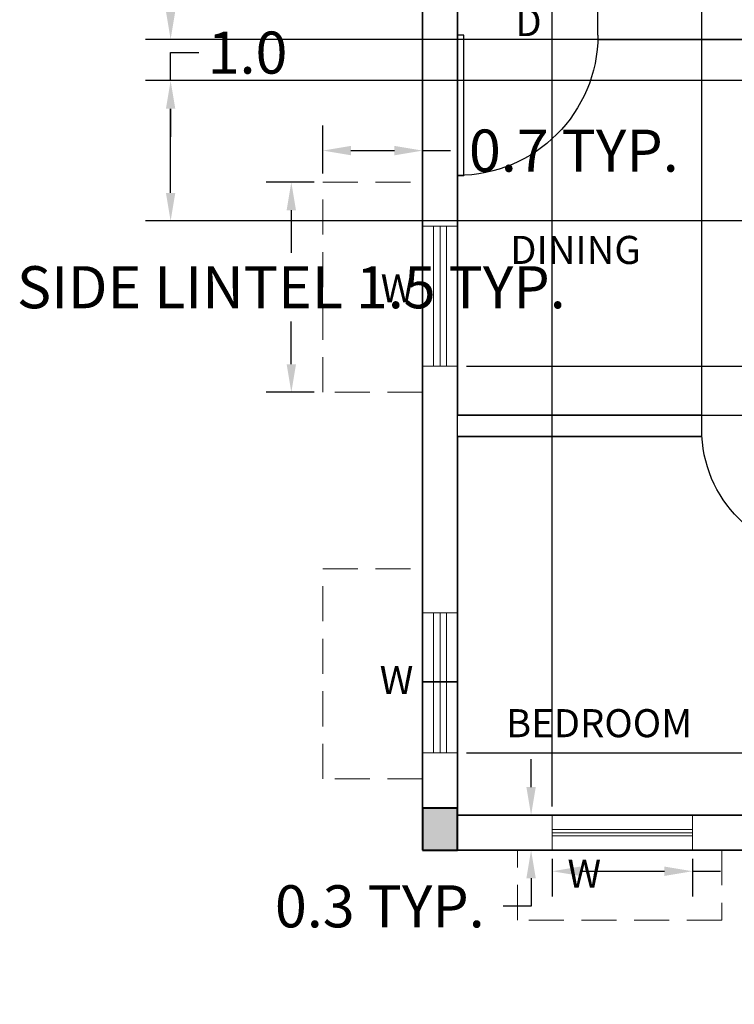
# Model space of a CAD drawing. Units: metres. Extents: x 106.5 to 121.4, y 89.1 to 111.8.
# Tile 1 of 5: x 107.3 to 112.4, y 90.2 to 97.3. Entities that reach past the tile are written whole.
import ezdxf

# ---------------------------------------------------------------- set-up
doc = ezdxf.new("R2010")
doc.units = ezdxf.units.M
doc.header["$MEASUREMENT"] = 0
doc.linetypes.add('HIDDEN', pattern=[0.375, 0.25, -0.125])
doc.layers.get('0').update_dxf_attribs({"color": 1})
for name, color, linetype, lineweight in [('A-ANNO-DIMS', 5, 'Continuous', 18), ('A-ANNO-TEXT', 4, 'Continuous', 18), ('A-AREA-IDEN', 4, 'Continuous', 18), ('A-COLS-PATT', 18, 'Continuous', 13), ('A-WALL', 1, 'Continuous', 35), ('COLUMN', 244, 'Continuous', 40), ('DR', 2, 'Continuous', 25), ('LNTL', 240, 'HIDDEN', 18), ('WNDW', 3, 'Continuous', 18)]:
    doc.layers.add(name, color=color, linetype=linetype, lineweight=lineweight)
doc.styles.get("Standard").update_dxf_attribs({"font": 'arial.ttf'})
doc.dimstyles.get("Standard").update_dxf_attribs({"dimtxt": 0.3, "dimasz": 0.2, "dimexe": 0.18, "dimexo": 0.0625, "dimgap": 0.09, "dimtad": 0, "dimtih": 1, "dimtoh": 1, "dimdec": 1, "dimzin": 0, "dimdsep": 46, "dimtxsty": 'Standard', "dimcen": 0.09, "dimadec": 0, "dimazin": 0, "dimtfac": 1, "dimtdec": 1, "dimtofl": 0, "dimtmove": 0, "dimatfit": 3, "dimfxl": 1, "dimtolj": 1, "dimtzin": 0, "dimarcsym": 0})

# ---------------------------------------------------------------- blocks, each defined once
blk = doc.blocks.new('*U2')
for p, q in [((0, 0), (0, -100)), ((-900, 0), (-900, -100))]:
    blk.add_line(p, q)
blk.add_lwpolyline([(0, 0), (0, 900), (-43.75, 900), (-43.75, 0)], close=True)
blk.add_arc((0, 0), 900, 90, 180)
blk = doc.blocks.new('*U5')
for p, q in [((0, 0), (0, -100)), ((1000, 0), (1000, -100))]:
    blk.add_line(p, q)
blk.add_lwpolyline([(0, 0), (0, 1000), (43.75, 1000), (43.75, 0)], close=True)
blk.add_arc((0, 0), 1000, 0, 90)
blk = doc.blocks.new('WIN-1000-SIDE')
for p, q in [((0.0782, 0.9998), (0.0782, -0.0002)), ((0.1249, 0.9998), (0.1249, -0.0002)), ((0.1718, -0.0002), (0.1718, 0.9998))]:
    blk.add_line(p, q)
blk.add_lwpolyline([(-0.0001, 0.9998), (0.2499, 0.9998), (0.2499, -0.0002), (-0.0001, -0.0002)], close=True)
blk = doc.blocks.new('WIN-1000-END')
for p, q in [((-0.0003, 0.1472), (0.9997, 0.1472)), ((-0.0003, 0.1248), (0.9997, 0.1248)), ((-0.0003, 0.1026), (0.9997, 0.1026))]:
    blk.add_line(p, q)
blk.add_lwpolyline([(-0.0003, 0.2498), (0.9997, 0.2498), (0.9997, -0.0002), (-0.0003, -0.0002)], close=True)
blk = doc.blocks.new('LINTEL-PROJ-1498')
for p, q in [((0.0003, -0.0001), (0.0003, 1.4981)), ((0.0003, 1.4981), (0.7109, 1.4981)), ((0.7109, -0.0001), (0.0003, -0.0001))]:
    blk.add_line(p, q)
blk = doc.blocks.new('LINTEL-PROJ-1456')
for p, q in [((0.0005, -0.0002), (0.0005, 0.4976)), ((0.0005, 0.4976), (1.4557, 0.4976)), ((1.4557, 0.4976), (1.4557, -0.0002))]:
    blk.add_line(p, q)
blk = doc.blocks.new('COL-250X300')
at = {"ltscale": 0.5}
blk.add_lwpolyline([(-0.0001, 0.2999), (0.2499, 0.2999), (0.2499, -0.0001), (-0.0001, -0.0001)], close=True, dxfattribs=at)
blk = doc.blocks.new('*D40')
at = {"layer": 'A-ANNO-DIMS', "color": 0, "lineweight": -2, "ltscale": 0.5, "transparency": 16777216}
for p, q in [((111.1267, 91.2713), (111.1267, 91.0038)), ((112.1267, 91.2713), (112.1267, 91.0038)), ((111.3267, 91.1838), (111.9267, 91.1838)), ((112.1267, 91.1838), (112.3267, 91.1838))]:
    blk.add_line(p, q, dxfattribs=at)
at = {"layer": 'A-ANNO-DIMS', "color": 0, "lineweight": -3, "ltscale": 0.5, "transparency": 16777216}
for points in [[(111.3267, 91.2171), (111.3267, 91.1505), (111.1267, 91.1838)], [(111.9267, 91.2171), (111.9267, 91.1505), (112.1267, 91.1838)]]:
    blk.add_solid(points, dxfattribs=at)
at = {"layer": 'Defpoints', "color": 0, "lineweight": -3, "ltscale": 0.5, "transparency": 16777216}
for p in [(111.1267, 91.3338), (112.1267, 91.3338), (112.1267, 91.1838)]:
    blk.add_point(p, dxfattribs=at)
at = {"layer": 'A-ANNO-DIMS', "color": 0, "ltscale": 0.5, "transparency": 16777216, "insert": (114.6755, 91.1838), "char_height": 0.3, "attachment_point": 5}
blk.add_mtext('\\A1;END WINDOW 1.0 TYP.', dxfattribs=at)
blk = doc.blocks.new('*D41')
at = {"layer": 'A-ANNO-DIMS', "color": 0, "lineweight": -2, "ltscale": 0.5, "transparency": 16777216}
for p, q in [((110.9767, 91.7838), (110.9767, 91.9838)), ((111.0642, 91.5838), (110.7967, 91.5838)), ((111.0642, 91.3338), (110.7967, 91.3338)), ((110.9767, 91.1338), (110.9767, 90.9338)), ((110.9767, 90.9338), (110.7767, 90.9338))]:
    blk.add_line(p, q, dxfattribs=at)
at = {"layer": 'A-ANNO-DIMS', "color": 0, "lineweight": -3, "ltscale": 0.5, "transparency": 16777216}
for points in [[(110.9433, 91.7838), (111.01, 91.7838), (110.9767, 91.5838)], [(110.9433, 91.1338), (111.01, 91.1338), (110.9767, 91.3338)]]:
    blk.add_solid(points, dxfattribs=at)
at = {"layer": 'Defpoints', "color": 0, "lineweight": -3, "ltscale": 0.5, "transparency": 16777216}
for p in [(111.1267, 91.5838), (110.9767, 91.3338), (111.1267, 91.3338)]:
    blk.add_point(p, dxfattribs=at)
at = {"layer": 'A-ANNO-DIMS', "color": 0, "ltscale": 0.5, "transparency": 16777216, "insert": (109.8983, 90.9338), "char_height": 0.3, "attachment_point": 5}
blk.add_mtext('\\A1;0.3 TYP.', dxfattribs=at)
blk = doc.blocks.new('*D48')
at = {"layer": 'A-ANNO-DIMS', "color": 0, "lineweight": -2, "ltscale": 0.5, "transparency": 16777216}
for p, q in [((109.4298, 96.0958), (109.0875, 96.0958)), ((109.2675, 95.8958), (109.2675, 95.5918)), ((109.2675, 94.7976), (109.2675, 95.1016)), ((109.4298, 94.5976), (109.0875, 94.5976))]:
    blk.add_line(p, q, dxfattribs=at)
at = {"layer": 'A-ANNO-DIMS', "color": 0, "lineweight": -3, "ltscale": 0.5, "transparency": 16777216}
for points in [[(109.2342, 95.8958), (109.3009, 95.8958), (109.2675, 96.0958)], [(109.2342, 94.7976), (109.3009, 94.7976), (109.2675, 94.5976)]]:
    blk.add_solid(points, dxfattribs=at)
at = {"layer": 'Defpoints', "color": 0, "lineweight": -3, "ltscale": 0.5, "transparency": 16777216}
for p in [(109.2675, 96.0958), (109.4923, 96.0958), (109.4923, 94.5976)]:
    blk.add_point(p, dxfattribs=at)
at = {"layer": 'A-ANNO-DIMS', "color": 0, "ltscale": 0.5, "transparency": 16777216, "insert": (109.2675, 95.3467), "char_height": 0.3, "attachment_point": 5}
blk.add_mtext('\\A1;SIDE LINTEL 1.5 TYP.', dxfattribs=at)
blk = doc.blocks.new('*D49')
at = {"layer": 'A-ANNO-DIMS', "color": 0, "lineweight": -2, "ltscale": 0.5, "transparency": 16777216}
for p, q in [((109.4923, 96.1583), (109.4923, 96.5006)), ((110.2029, 96.1583), (110.2029, 96.5006)), ((109.6923, 96.3206), (110.0029, 96.3206)), ((110.2029, 96.3206), (110.4029, 96.3206))]:
    blk.add_line(p, q, dxfattribs=at)
at = {"layer": 'A-ANNO-DIMS', "color": 0, "lineweight": -3, "ltscale": 0.5, "transparency": 16777216}
for points in [[(109.6923, 96.3539), (109.6923, 96.2872), (109.4923, 96.3206)], [(110.0029, 96.3539), (110.0029, 96.2872), (110.2029, 96.3206)]]:
    blk.add_solid(points, dxfattribs=at)
at = {"layer": 'Defpoints', "color": 0, "lineweight": -3, "ltscale": 0.5, "transparency": 16777216}
for p in [(110.2029, 96.3206), (109.4923, 96.0958), (110.2029, 96.0958)]:
    blk.add_point(p, dxfattribs=at)
at = {"layer": 'A-ANNO-DIMS', "color": 0, "ltscale": 0.5, "transparency": 16777216, "insert": (111.2813, 96.3206), "char_height": 0.3, "attachment_point": 5}
blk.add_mtext('\\A1;0.7 TYP.', dxfattribs=at)
blk = doc.blocks.new('*D58')
at = {"layer": 'A-ANNO-DIMS', "color": 0, "lineweight": -2, "ltscale": 0.5, "transparency": 16777216}
for p, q in [((110.4529, 97.2063), (110.4529, 111.7688)), ((111.4529, 97.1762), (111.4529, 111.7688)), ((110.2529, 111.5888), (110.0529, 111.5888)), ((111.6529, 111.5888), (111.8529, 111.5888))]:
    blk.add_line(p, q, dxfattribs=at)
at = {"layer": 'A-ANNO-DIMS', "color": 0, "lineweight": -3, "ltscale": 0.5, "transparency": 16777216}
for points in [[(110.2529, 111.6221), (110.2529, 111.5555), (110.4529, 111.5888)], [(111.6529, 111.6221), (111.6529, 111.5555), (111.4529, 111.5888)]]:
    blk.add_solid(points, dxfattribs=at)
at = {"layer": 'Defpoints', "color": 0, "lineweight": -3, "ltscale": 0.5, "transparency": 16777216}
for p in [(111.4529, 111.5888), (110.4529, 97.1438), (111.4529, 97.1137)]:
    blk.add_point(p, dxfattribs=at)
at = {"layer": 'A-ANNO-DIMS', "color": 0, "ltscale": 0.5, "transparency": 16777216, "insert": (110.9529, 111.5888), "char_height": 0.3, "attachment_point": 5}
blk.add_mtext('\\A1;1.0', dxfattribs=at)
blk = doc.blocks.new('*D59')
at = {"layer": 'A-ANNO-DIMS', "color": 0, "lineweight": -2, "ltscale": 0.5, "transparency": 16777216}
for p, q in [((112.1943, 94.3463), (112.1943, 111.7688)), ((113.0929, 94.3463), (113.0929, 111.7688)), ((112.3943, 111.5888), (112.8929, 111.5888)), ((113.0929, 111.5888), (113.2929, 111.5888))]:
    blk.add_line(p, q, dxfattribs=at)
at = {"layer": 'A-ANNO-DIMS', "color": 0, "lineweight": -3, "ltscale": 0.5, "transparency": 16777216}
for points in [[(112.3943, 111.6221), (112.3943, 111.5555), (112.1943, 111.5888)], [(112.8929, 111.6221), (112.8929, 111.5555), (113.0929, 111.5888)]]:
    blk.add_solid(points, dxfattribs=at)
at = {"layer": 'Defpoints', "color": 0, "lineweight": -3, "ltscale": 0.5, "transparency": 16777216}
for p in [(113.0929, 111.5888), (112.1943, 94.2838), (113.0929, 94.2838)]:
    blk.add_point(p, dxfattribs=at)
at = {"layer": 'A-ANNO-DIMS', "color": 0, "ltscale": 0.5, "transparency": 16777216, "insert": (113.772, 111.5888), "char_height": 0.3, "attachment_point": 5}
blk.add_mtext('\\A1;0.90', dxfattribs=at)
blk = doc.blocks.new('*D63')
at = {"layer": 'A-ANNO-DIMS', "color": 0, "lineweight": -2, "ltscale": 0.5, "transparency": 16777216}
for p, q in [((110.4529, 91.6463), (110.4529, 111.7688)), ((111.1267, 91.6463), (111.1267, 111.7688)), ((110.6529, 111.5888), (110.9267, 111.5888)), ((111.1267, 111.5888), (111.3267, 111.5888))]:
    blk.add_line(p, q, dxfattribs=at)
at = {"layer": 'A-ANNO-DIMS', "color": 0, "lineweight": -3, "ltscale": 0.5, "transparency": 16777216}
for points in [[(110.6529, 111.6221), (110.6529, 111.5555), (110.4529, 111.5888)], [(110.9267, 111.6221), (110.9267, 111.5555), (111.1267, 111.5888)]]:
    blk.add_solid(points, dxfattribs=at)
at = {"layer": 'Defpoints', "color": 0, "lineweight": -3, "ltscale": 0.5, "transparency": 16777216}
for p in [(111.1267, 111.5888), (110.4529, 91.5838), (111.1267, 91.5838)]:
    blk.add_point(p, dxfattribs=at)
at = {"layer": 'A-ANNO-DIMS', "color": 0, "ltscale": 0.5, "transparency": 16777216, "insert": (111.8063, 111.5888), "char_height": 0.3, "attachment_point": 5}
blk.add_mtext('\\A1;0.67', dxfattribs=at)
blk = doc.blocks.new('*D67')
at = {"layer": 'A-ANNO-DIMS', "color": 0, "lineweight": -2, "ltscale": 0.5, "transparency": 16777216}
for p, q in [((119.3535, 92.2268), (119.3535, 92.4268)), ((119.3535, 92.4268), (119.5535, 92.4268)), ((110.5154, 92.0268), (119.5335, 92.0268)), ((110.5154, 91.5838), (119.5335, 91.5838)), ((119.3535, 91.3838), (119.3535, 91.1838))]:
    blk.add_line(p, q, dxfattribs=at)
at = {"layer": 'A-ANNO-DIMS', "color": 0, "lineweight": -3, "ltscale": 0.5, "transparency": 16777216}
for points in [[(119.3201, 92.2268), (119.3868, 92.2268), (119.3535, 92.0268)], [(119.3201, 91.3838), (119.3868, 91.3838), (119.3535, 91.5838)]]:
    blk.add_solid(points, dxfattribs=at)
at = {"layer": 'Defpoints', "color": 0, "lineweight": -3, "ltscale": 0.5, "transparency": 16777216}
for p in [(110.4529, 92.0268), (119.3535, 92.0268), (110.4529, 91.5838)]:
    blk.add_point(p, dxfattribs=at)
at = {"layer": 'A-ANNO-DIMS', "color": 0, "ltscale": 0.5, "transparency": 16777216, "insert": (120.1496, 92.4268), "char_height": 0.3, "attachment_point": 5}
blk.add_mtext('\\A1;0.443', dxfattribs=at)
blk = doc.blocks.new('*D68')
at = {"layer": 'A-ANNO-DIMS', "color": 0, "lineweight": -2, "ltscale": 0.5, "transparency": 16777216}
for p, q in [((119.3535, 94.9829), (119.3535, 95.1829)), ((119.3535, 95.1829), (119.5535, 95.1829)), ((110.5154, 94.7829), (119.5335, 94.7829)), ((110.5154, 94.4338), (119.5335, 94.4338)), ((119.3535, 94.2338), (119.3535, 94.0338))]:
    blk.add_line(p, q, dxfattribs=at)
at = {"layer": 'A-ANNO-DIMS', "color": 0, "lineweight": -3, "ltscale": 0.5, "transparency": 16777216}
for points in [[(119.3201, 94.9829), (119.3868, 94.9829), (119.3535, 94.7829)], [(119.3201, 94.2338), (119.3868, 94.2338), (119.3535, 94.4338)]]:
    blk.add_solid(points, dxfattribs=at)
at = {"layer": 'Defpoints', "color": 0, "lineweight": -3, "ltscale": 0.5, "transparency": 16777216}
for p in [(110.4529, 94.7829), (119.3535, 94.7829), (110.4529, 94.4338)]:
    blk.add_point(p, dxfattribs=at)
at = {"layer": 'A-ANNO-DIMS', "color": 0, "ltscale": 0.5, "transparency": 16777216, "insert": (120.0342, 95.1829), "char_height": 0.3, "attachment_point": 5}
blk.add_mtext('\\A1;0.35', dxfattribs=at)
blk = doc.blocks.new('*D69')
at = {"layer": 'A-ANNO-DIMS', "color": 0, "lineweight": -2, "ltscale": 0.5, "transparency": 16777216}
for p, q in [((108.4073, 97.3137), (108.4073, 97.5137)), ((108.4073, 97.5137), (108.6073, 97.5137)), ((117.4704, 97.1137), (108.2273, 97.1137)), ((117.4697, 96.8192), (108.2273, 96.8192)), ((108.4073, 96.6192), (108.4073, 96.4192))]:
    blk.add_line(p, q, dxfattribs=at)
at = {"layer": 'A-ANNO-DIMS', "color": 0, "lineweight": -3, "ltscale": 0.5, "transparency": 16777216}
for points in [[(108.3739, 97.3137), (108.4406, 97.3137), (108.4073, 97.1137)], [(108.3739, 96.6192), (108.4406, 96.6192), (108.4073, 96.8192)]]:
    blk.add_solid(points, dxfattribs=at)
at = {"layer": 'Defpoints', "color": 0, "lineweight": -3, "ltscale": 0.5, "transparency": 16777216}
for p in [(108.4073, 97.1137), (117.5329, 97.1137), (117.5322, 96.8192)]:
    blk.add_point(p, dxfattribs=at)
at = {"layer": 'A-ANNO-DIMS', "color": 0, "ltscale": 0.5, "transparency": 16777216, "insert": (109.0872, 97.5137), "char_height": 0.3, "attachment_point": 5}
blk.add_mtext('\\A1;0.29', dxfattribs=at)
blk = doc.blocks.new('*D70')
at = {"layer": 'A-ANNO-DIMS', "color": 0, "lineweight": -2, "ltscale": 0.5, "transparency": 16777216}
for p, q in [((108.4073, 96.8192), (108.4073, 97.0191)), ((108.4073, 97.0191), (108.6073, 97.0191)), ((117.4697, 96.8192), (108.2273, 96.8192)), ((108.4073, 96.0192), (108.4073, 96.6192)), ((117.4697, 95.8192), (108.2273, 95.8192))]:
    blk.add_line(p, q, dxfattribs=at)
at = {"layer": 'A-ANNO-DIMS', "color": 0, "lineweight": -3, "ltscale": 0.5, "transparency": 16777216}
for points in [[(108.3739, 96.6192), (108.4406, 96.6192), (108.4073, 96.8192)], [(108.3739, 96.0192), (108.4406, 96.0192), (108.4073, 95.8192)]]:
    blk.add_solid(points, dxfattribs=at)
at = {"layer": 'Defpoints', "color": 0, "lineweight": -3, "ltscale": 0.5, "transparency": 16777216}
for p in [(108.4073, 96.8192), (117.5322, 96.8192), (117.5322, 95.8192)]:
    blk.add_point(p, dxfattribs=at)
at = {"layer": 'A-ANNO-DIMS', "color": 0, "ltscale": 0.5, "transparency": 16777216, "insert": (108.9557, 97.0191), "char_height": 0.3, "attachment_point": 5}
blk.add_mtext('\\A1;1.0', dxfattribs=at)

msp = doc.modelspace()

# ---------------------------------------------------------------- hatches: boundary and pattern name
at = {"layer": 'A-COLS-PATT', "ltscale": 0.5}
h = msp.add_hatch(color=256, dxfattribs=at)
h.dxf.hatch_style = 1
h.paths.add_polyline_path([(110.4529, 103.8929), (110.2029, 103.8929), (110.2029, 103.5938), (110.4529, 103.5938)])
h.paths.add_polyline_path([(114.4629, 103.8938), (114.3632, 103.8938), (114.3632, 103.7438), (114.4629, 103.7438)])
h.paths.add_polyline_path([(114.6129, 103.8938), (114.4629, 103.8938), (114.4629, 103.7438), (114.6129, 103.7438)])
h.paths.add_polyline_path([(114.6132, 103.7438), (114.4629, 103.7438), (114.3632, 103.7438), (114.3632, 103.5938), (114.6132, 103.5938)])
h.paths.add_polyline_path([(117.7829, 103.8996), (117.5329, 103.8996), (117.5329, 103.5996), (117.7829, 103.5996)])
h.paths.add_polyline_path([(117.7829, 98.888), (117.5329, 98.888), (117.5329, 98.588), (117.7829, 98.588)])
h.paths.add_polyline_path([(110.4529, 98.8938), (110.2029, 98.8938), (110.2029, 98.5947), (110.4529, 98.5947)])
h.paths.add_polyline_path([(114.6132, 98.8938), (114.3132, 98.8938), (114.3132, 98.7438), (114.4632, 98.7438), (114.6132, 98.7438)])
h.paths.add_polyline_path([(110.4529, 91.6338), (110.2029, 91.6338), (110.2029, 91.3338), (110.4529, 91.3338)])
h.paths.add_polyline_path([(114.6132, 91.5838), (114.6129, 91.5838), (114.6129, 91.6338), (114.4629, 91.6338), (114.4629, 91.5838), (114.3632, 91.5838), (114.3632, 91.3338), (114.6132, 91.3338)])
h.paths.add_polyline_path([(117.7821, 91.6338), (117.5329, 91.6338), (117.5329, 91.5838), (117.5321, 91.3338), (117.7821, 91.3338)])
h = msp.add_hatch(dxfattribs=at)
h.set_pattern_fill('CORK', color=256, scale=10)
h.set_pattern_definition([(0, (0, 0), (0, 1.25), []), (135, (0.625, -0.625), (-2.5, -2.5), [1.76777, -1.76777]), (135, (0.9375, -0.625), (-2.5, -2.5), [1.76777, -1.76777]), (135, (1.25, -0.625), (-2.5, -2.5), [1.76777, -1.76777])])
h.paths.add_polyline_path([(110.2029, 93.2238), (110.2029, 93.5238), (110.4529, 93.5238), (110.4529, 93.2238)])
h.paths.add_polyline_path([(114.6132, 93.2238), (114.3632, 93.2238), (114.3632, 93.4738), (114.4629, 93.4738), (114.4629, 93.5238), (114.6129, 93.5238), (114.6129, 93.4738)])
h.paths.add_polyline_path([(117.5321, 93.4738), (117.5329, 93.4738), (117.5329, 93.5238), (117.7821, 93.5238), (117.7821, 93.2238), (117.5321, 93.2238)])

# ---------------------------------------------------------------- linework, layer by layer
at = {"layer": 'A-WALL'}
for p, q in [((110.2029, 91.3338), (110.2029, 101.9438)), ((110.4529, 94.4338), (110.4529, 98.5947)), ((114.4629, 97.1137), (111.4529, 97.1137)), ((112.1929, 94.4338), (110.4529, 94.4338)), ((112.1943, 94.2838), (110.4529, 94.2838)), ((110.4529, 91.5838), (110.4529, 94.2838)), ((110.2029, 92.5338), (110.4529, 92.5338)), ((113.0929, 91.5838), (110.4529, 91.5838)), ((117.7829, 91.3338), (110.2029, 91.3338))]:
    msp.add_line(p, q, dxfattribs=at)

# ---------------------------------------------------------------- block references
at = {"layer": 'COLUMN', "extrusion": (0, 0, -1), "zscale": -1, "rotation": 180}
msp.add_blockref('COL-250X300', (-110.203, 91.6337), dxfattribs=at)
at = {"layer": 'DR', "xscale": -0.001, "yscale": 0.001, "zscale": 0.001, "rotation": 180}
for name, p in [('*U5', (110.4529, 97.1438)), ('*U2', (113.0929, 94.3338))]:
    msp.add_blockref(name, p, dxfattribs=at)
at = {"layer": 'LNTL'}
for p in [(109.492, 94.5977), (109.492, 91.8416)]:
    msp.add_blockref('LINTEL-PROJ-1498', p, dxfattribs=at)
at = {"layer": 'LNTL', "rotation": 180}
msp.add_blockref('LINTEL-PROJ-1456', (112.3362, 91.3336), dxfattribs=at)
at = {"layer": 'WNDW', "extrusion": (0, 0, -1), "zscale": -1, "rotation": 180}
for name, p in [('WIN-1000-SIDE', (-110.203, 95.7828)), ('WIN-1000-SIDE', (-110.203, 93.0266)), ('WIN-1000-END', (-111.127, 91.5836))]:
    msp.add_blockref(name, p, dxfattribs=at)

# ---------------------------------------------------------------- texts
at = {"layer": 'A-ANNO-TEXT', "ltscale": 0.5, "char_height": 0.2}
for s, width, insert, attachment_point in [('D', 0.320447, (110.8641, 97.3364), 1), ('W', 0.390771, (109.9045, 95.2388), 7), ('W', 0.390771, (109.8975, 92.4462), 7), ('W', 0.390771, (111.2359, 91.066), 7)]:
    msp.add_mtext_dynamic_manual_height_columns(s, width=width, gutter_width=1, heights=[0], dxfattribs=dict(at, insert=insert, attachment_point=attachment_point))
at = {"layer": 'A-AREA-IDEN', "ltscale": 0.5, "char_height": 0.2, "attachment_point": 7}
for s, insert in [('DINING', (110.8277, 95.5127)), ('BEDROOM', (110.7979, 92.1393))]:
    msp.add_mtext_dynamic_manual_height_columns(s, width=0.914899, gutter_width=1, heights=[0], dxfattribs=dict(at, insert=insert))

# ---------------------------------------------------------------- dimensions: what is measured, and where the dimension line sits
at = {"layer": 'A-ANNO-DIMS', "ltscale": 0.5}
for base, p1, p2, override, picture, middle in [((111.4529, 111.5888), (110.4529, 97.1438), (111.4529, 97.1137), {"dimdec": 1, "dimlfac": 1, "dimrnd": 0, "dimzin": 0, "dimdsep": 46, "dimlunit": 2}, '*D58', (110.9529, 111.5888)), ((111.1267, 111.5888), (110.4529, 91.5838), (111.1267, 91.5838), {"dimdec": 2, "dimlfac": 1, "dimrnd": 0, "dimzin": 0, "dimdsep": 46, "dimlunit": 2}, '*D63', (111.8063, 111.5888)), ((113.0929, 111.5888), (112.1943, 94.2838), (113.0929, 94.2838), {"dimdec": 2, "dimlfac": 1, "dimrnd": 0, "dimzin": 0, "dimdsep": 46, "dimlunit": 2}, '*D59', (113.772, 111.5888))]:
    dim = msp.add_linear_dim(base=base, p1=p1, p2=p2, dimstyle='Standard', override=override, dxfattribs=at)
    dim.commit()
    dim.dimension.update_dxf_attribs({"geometry": picture, "text_midpoint": middle})
for base, p1, p2, override, picture, middle in [((108.4073, 97.1137), (117.5322, 96.8191), (117.5329, 97.1137), {"dimdec": 2, "dimlfac": 1, "dimrnd": 0, "dimzin": 0, "dimdsep": 46, "dimlunit": 2}, '*D69', (109.0872, 97.5137)), ((108.4073, 96.8191), (117.5322, 95.8191), (117.5322, 96.8191), {"dimdec": 1, "dimlfac": 1, "dimrnd": 0, "dimzin": 0, "dimdsep": 46, "dimlunit": 2}, '*D70', (108.9557, 97.0191)), ((119.3535, 94.7829), (110.4529, 94.4338), (110.4529, 94.7829), {"dimdec": 2, "dimlfac": 1, "dimrnd": 0, "dimzin": 0, "dimdsep": 46, "dimlunit": 2}, '*D68', (120.0342, 95.1829)), ((119.3535, 92.0268), (110.4529, 91.5838), (110.4529, 92.0268), {"dimdec": 3, "dimlfac": 1, "dimrnd": 0, "dimzin": 0, "dimdsep": 46, "dimlunit": 2}, '*D67', (120.1496, 92.4268))]:
    dim = msp.add_linear_dim(base=base, p1=p1, p2=p2, angle=90, dimstyle='Standard', override=override, dxfattribs=at)
    dim.commit()
    dim.dimension.update_dxf_attribs({"geometry": picture, "text_midpoint": middle})
for base, p1, p2, text, picture, middle in [((110.2029, 96.3206), (109.4923, 96.0958), (110.2029, 96.0958), '<> TYP.', '*D49', (111.2813, 96.3206)), ((112.1267, 91.1838), (111.1267, 91.3338), (112.1267, 91.3338), 'END WINDOW <> TYP.', '*D40', (114.6755, 91.1838))]:
    dim = msp.add_linear_dim(base=base, p1=p1, p2=p2, text=text, dimstyle='Standard', override={"dimdec": 1, "dimlfac": 1, "dimrnd": 0, "dimzin": 0, "dimdsep": 46, "dimlunit": 2}, dxfattribs=at)
    dim.commit()
    dim.dimension.update_dxf_attribs({"geometry": picture, "text_midpoint": middle})
for base, p1, p2, angle, text, picture, middle in [((109.2675, 96.0958), (109.4923, 94.5976), (109.4923, 96.0958), 90, 'SIDE LINTEL <> TYP.', '*D48', (109.2675, 95.3467)), ((110.9766554778, 91.3338026801), (111.1266554778, 91.5838026801), (111.1266554778, 91.3338026801), 270, '<> TYP.', '*D41', (109.8982857643, 90.9338026801))]:
    dim = msp.add_linear_dim(base=base, p1=p1, p2=p2, angle=angle, text=text, dimstyle='Standard', override={"dimdec": 1, "dimlfac": 1, "dimrnd": 0, "dimzin": 0, "dimdsep": 46, "dimlunit": 2}, dxfattribs=at)
    dim.commit()
    dim.dimension.update_dxf_attribs({"geometry": picture, "text_midpoint": middle})

doc.saveas('drawing.dxf')
